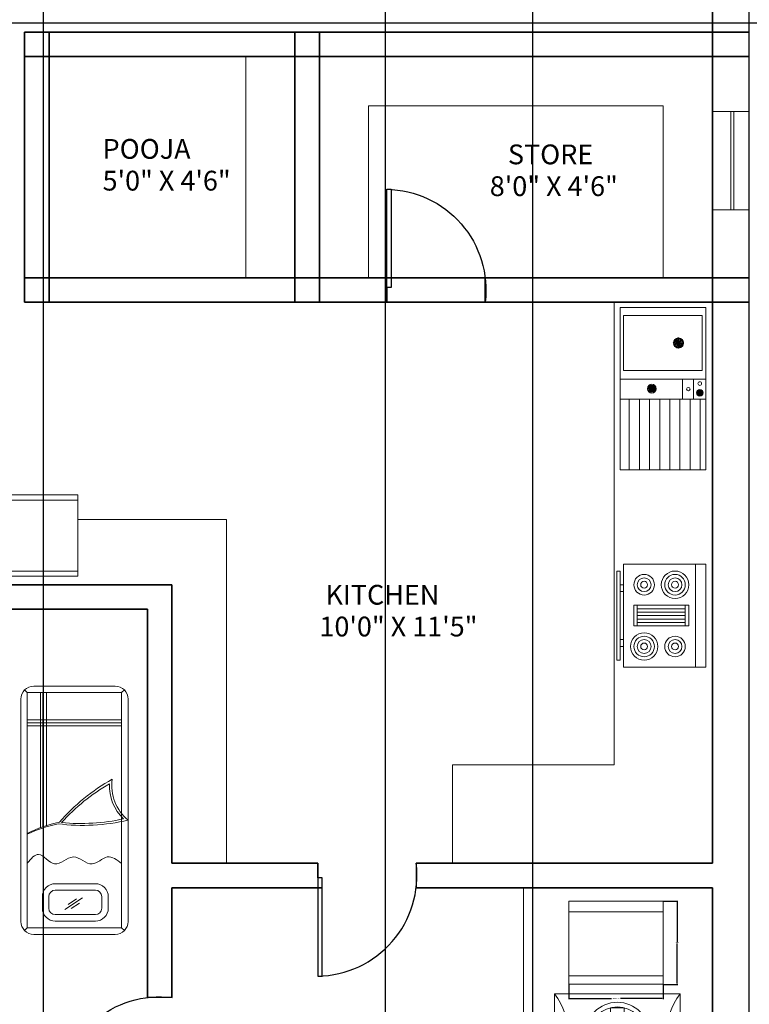
# Model space of a CAD drawing. Units: inches. Extents: x -61 to 1599, y -1316 to 257.
# Tile 94 of 204: x 367 to 545, y -407 to -166. Entities that reach past the tile are written whole.
import ezdxf

# ---------------------------------------------------------------- set-up
doc = ezdxf.new("R2010")
doc.units = ezdxf.units.IN
doc.header["$MEASUREMENT"] = 0
doc.linetypes.add('ACAD_ISO02W100', pattern=[15, 12, -3])
for name, color, linetype, lineweight in [('A-ANNO-DIMS', 2, 'Continuous', 18), ('A-AREA-IDEN', 1, 'Continuous', 18), ('A-EQPM', 9, 'Continuous', 18), ('A-FLOR-CASE', 8, 'Continuous', 18), ('A-FLOR-FIXT', 8, 'Continuous', 18), ('A-WALL-JAMB', 4, 'ACAD_ISO02W100', 25), ('DOORS', 2, 'Continuous', 25), ('FURNITURE', 83, 'Continuous', 18), ('WALLS', 4, 'Continuous', 35), ('WINDOWS', 220, 'Continuous', 18)]:
    doc.layers.add(name, color=color, linetype=linetype, lineweight=lineweight)
doc.layers.add('FUR', color=83, linetype='Continuous')
doc.styles.get("Standard").update_dxf_attribs({"font": 'arial.ttf'})
doc.dimstyles.get("Standard").update_dxf_attribs({"dimtxt": 0.18, "dimasz": 0.18, "dimexe": 0.18, "dimexo": 0.0625, "dimgap": 0.09, "dimtad": 0, "dimtih": 1, "dimtoh": 1, "dimdec": 0, "dimzin": 0, "dimdsep": 46, "dimlunit": 3, "dimtxsty": 'Standard', "dimcen": 0.09, "dimadec": 0, "dimazin": 0, "dimtfac": 1, "dimtdec": 0, "dimtofl": 0, "dimtmove": 0, "dimatfit": 3, "dimfxl": 1, "dimtolj": 1, "dimtzin": 0, "dimarcsym": 0})

# ---------------------------------------------------------------- blocks, each defined once
blk = doc.blocks.new('Range-Oven - 30 in top')
for p, q in [((0, -3), (30, -3)), ((12, -6), (18, -6)), ((13, -20), (13, -6)), ((14, -6), (14, -20)), ((15, -20), (15, -6)), ((16, -6), (16, -20)), ((17, -20), (17, -6)), ((18, -20), (12, -20)), ((6, -24), (6, -25)), ((8, -25), (8, -24)), ((22, -25), (22, -24)), ((24, -24), (24, -25))]:
    blk.add_line(p, q)
for points in [[(0, -24), (0, 0), (30, 0), (30, -24)], [(12, -21), (12, -5), (18, -5), (18, -21)], [(2, -26), (2, -25), (28, -25), (28, -26)]]:
    blk.add_lwpolyline(points, close=True)
for centre, radius in [((6, -9), 4), ((6, -9), 3), ((6, -9), 2), ((6, -9), 1), ((24, -9), 3), ((24, -9), 2), ((24, -9), 1), ((24, -18), 4), ((6, -18), 3), ((6, -18), 2), ((6, -18), 1), ((24, -18), 3), ((24, -18), 2), ((24, -18), 1)]:
    blk.add_circle(centre, radius)
blk = doc.blocks.new('DOOR-SWING-24')
blk.add_line((0, 0), (0, 3.6))
blk.add_lwpolyline([(0, 0), (0, -24), (1.05, -24), (1.05, 0)], close=True)
blk.add_arc((-0.44, 0.62), 24.62, 271.0259, 6.9559)
blk = doc.blocks.new('WIN-24IN')
for p, q in [((0, 4.5), (0, 9)), ((0, 9), (0, 0)), ((24, 9), (24, 0)), ((0, 5.19), (24, 5.19)), ((0, 4.5), (24, 4.5))]:
    blk.add_line(p, q)
blk = doc.blocks.new('*U268')
at = {"layer": 'FUR'}
blk.add_line((0.41, 1.36), (0.41, 0.68), dxfattribs=at)
blk.add_open_spline([(0.41, 1.36), (0.24, 1.25), (-0.09, 1.02), (0.41, 0.7), (0.83, 0.34), (0.55, 0.11), (0.41, 0)], degree=3, knots=[0, 0, 0, 0, 0.474547, 0.949094, 1.393355, 1.837616, 1.837616, 1.837616, 1.837616], dxfattribs=at)
blk = doc.blocks.new('*U269')
at = {"layer": 'FUR', "transparency": 16777216}
for p, rotation in [((531.82, -257.55), 308.5714285714286), ((532.89, -258.18), 51.42857142857144), ((532.03, -256.89), 257.1428571428571), ((533.36, -257.68), 102.8571428571428), ((532.68, -256.65), 205.7142857142857), ((533.27, -257), 154.2857142857143)]:
    blk.add_blockref('*U268', p, dxfattribs=dict(at, rotation=rotation))
blk.add_blockref('*U268', (532.2, -258.12), dxfattribs=at)
blk = doc.blocks.new('*U270')
at = {"layer": 'FUR'}
blk.add_line((0.74, 2.46), (0.74, 1.23), dxfattribs=at)
blk.add_open_spline([(0.74, 2.46), (0.44, 2.26), (-0.16, 1.84), (0.74, 1.26), (1.5, 0.61), (0.99, 0.2), (0.74, 0)], degree=3, knots=[0, 0, 0, 0, 0.85637, 1.712739, 2.514455, 3.316171, 3.316171, 3.316171, 3.316171], dxfattribs=at)
blk = doc.blocks.new('*U271')
at = {"layer": 'FUR', "transparency": 16777216}
for p, rotation in [((959.72, -464.77), 308.5714285714286), ((961.65, -465.92), 51.42857142857144), ((960.11, -463.59), 257.1428571428571), ((962.51, -465.02), 102.8571428571428), ((961.27, -463.15), 205.7142857142858), ((962.34, -463.79), 154.2857142857143)]:
    blk.add_blockref('*U270', p, dxfattribs=dict(at, rotation=rotation))
blk.add_blockref('*U270', (960.41, -465.81), dxfattribs=at)
blk = doc.blocks.new('*U266')
at = {"layer": 'FUR'}
blk.add_line((0.41, 1.36), (0.41, 0.68), dxfattribs=at)
blk.add_open_spline([(0.41, 1.36), (0.24, 1.25), (-0.09, 1.02), (0.41, 0.7), (0.83, 0.34), (0.55, 0.11), (0.41, 0)], degree=3, knots=[0, 0, 0, 0, 0.474547, 0.949094, 1.393355, 1.837616, 1.837616, 1.837616, 1.837616], dxfattribs=at)
blk = doc.blocks.new('*U267')
at = {"layer": 'FUR', "transparency": 16777216}
for p, rotation in [((531.82, -257.55), 308.5714285714286), ((532.89, -258.18), 51.42857142857144), ((532.03, -256.89), 257.1428571428571), ((533.36, -257.68), 102.8571428571428), ((532.68, -256.65), 205.7142857142857), ((533.27, -257), 154.2857142857143)]:
    blk.add_blockref('*U266', p, dxfattribs=dict(at, rotation=rotation))
blk.add_blockref('*U266', (532.2, -258.12), dxfattribs=at)
blk = doc.blocks.new('SINK-WITH-DRAINBOARD')
for p, q in [((14.29, 30.97), (14.29, 29.74)), ((0, 22.17), (20.98, 22.17)), ((15.24, 17.27), (15.24, 22.17)), ((17.97, 22.17), (17.97, 17.27)), ((7.79, 19.82), (7.79, 19.14)), ((0, 17.27), (20.98, 17.27)), ((2.27, 0), (2.27, 17.27)), ((4.74, 0), (4.74, 17.27)), ((7.21, 0), (7.21, 17.27)), ((9.69, 0), (9.69, 17.27)), ((12.16, 0), (12.16, 17.27)), ((14.63, 0), (14.63, 17.27)), ((17.1, 0), (17.1, 17.27)), ((19.48, 18.8), (19.48, 18.12)), ((19.58, 0), (19.58, 17.27))]:
    blk.add_line(p, q)
for points in [[(20.98, 0), (0, 0), (0, 39.63), (20.98, 39.63)], [(20.07, 24.22), (0.86, 24.22), (0.86, 37.7), (20.07, 37.7)]]:
    blk.add_lwpolyline(points, close=True)
for centre, radius in [((14.29, 30.97), 1.23), ((7.78, 19.81), 1.08), ((7.78, 19.81), 0.877), ((7.79, 19.82), 0.682), ((16.69, 19.72), 0.419), ((19.48, 18.8), 0.816), ((19.48, 18.8), 0.816), ((19.48, 18.8), 0.682), ((19.48, 21.05), 0.455)]:
    blk.add_circle(centre, radius)
for name, p in [('*U271', (-946.85, 495.54)), ('*U269', (-524.82, 277.26)), ('*U267', (-513.12, 276.24))]:
    blk.add_blockref(name, p)
blk = doc.blocks.new('WASHING-MACHINE')
for p, q in [((19.24, 4.47), (19.22, 15.41)), ((0.98, 10.64), (0.75, 10.64)), ((0.96, 11.16), (1.13, 11)), ((1.12, 10.28), (0.96, 10.12)), ((1.49, 11.38), (1.49, 11.15)), ((1.49, 10.12), (1.49, 9.89)), ((2.02, 11.15), (1.86, 10.99)), ((1.86, 10.28), (2.02, 10.12)), ((2.23, 10.64), (2, 10.64)), ((11, 9.47), (11, 11.68))]:
    blk.add_line(p, q)
for points in [[(30.68, 0), (0, 0), (0, 19.87), (30.68, 19.87)], [(16.98, 3.42), (13.7, 3.42), (13.7, 16.45), (16.98, 16.45)], [(20.43, 13.78), (18.01, 13.78), (18.01, 13.95), (20.43, 13.95)], [(18.09, 12.45), (20.41, 11.74), (20.35, 11.57), (18.04, 12.29)], [(18.21, 13.64), (20.52, 12.92), (20.47, 12.76), (18.16, 13.47)], [(18.22, 12.89), (20.53, 12.18), (20.48, 12.01), (18.17, 12.73)], [(20.44, 10.23), (18.02, 10.23), (18.02, 10.4), (20.44, 10.4)], [(18.1, 11.71), (20.41, 10.99), (20.36, 10.83), (18.05, 11.54)], [(18.22, 10.09), (20.53, 9.38), (20.48, 9.21), (18.17, 9.92)], [(18.1, 8.63), (20.42, 7.91), (20.37, 7.75), (18.05, 8.46)], [(18.11, 7.88), (20.42, 7.17), (20.37, 7), (18.06, 7.72)], [(18.23, 9.07), (20.54, 8.36), (20.49, 8.19), (18.18, 8.91)], [(20.45, 6.56), (18.03, 6.56), (18.03, 6.73), (20.45, 6.73)], [(18.23, 6.42), (20.54, 5.7), (20.49, 5.54), (18.18, 6.25)]]:
    blk.add_lwpolyline(points, close=True)
for centre, radius in [((15.34, 9.94), 7.85), ((15.34, 9.94), 7.85), ((15.34, 9.94), 6.71), ((1.28, 13.83), 0.526), ((10.77, 12.86), 0.381), ((10.77, 12.86), 0.289), ((1.49, 10.64), 0.742), ((1.49, 10.64), 0.513), ((1.49, 10.64), 0.178), ((1.49, 10.64), 0.07), ((1.28, 7.75), 0.526), ((10.77, 8.29), 0.381), ((10.77, 8.29), 0.289)]:
    blk.add_circle(centre, radius)
for centre, radius, start, end in [((-13.12, 9.94), 16.46, 322.8671, 37.1329), ((43.8, 9.94), 16.46, 142.8671, 217.1329), ((12.8, 10.57), 2.11, 148.4251, 211.5749), ((9.2, 10.57), 2.11, 328.4251, 31.5749)]:
    blk.add_arc(centre, radius, start, end)
blk = doc.blocks.new('UTILITY-CABINET')
for p, q in [((0, 17.69), (23.01, 17.69)), ((0, 2.1), (23.01, 2.1))]:
    blk.add_line(p, q)
blk.add_lwpolyline([(23.01, 0), (0, 0), (0, 20.31), (23.01, 20.31)], close=True)
blk = doc.blocks.new('KITCHEN-BASE-UNIT')
for p, q in [((25.07, 18.6), (0, 18.6)), ((25.07, 1.23), (0, 1.23))]:
    blk.add_line(p, q)
blk.add_lwpolyline([(25.07, 0), (0, 0), (0, 19.92), (25.07, 19.92)], close=True)
blk = doc.blocks.new('STORE-SHELVING')
for p, q in [((0, 42), (72, 42)), ((0, 12), (0, 42)), ((72, 42), (72, 12)), ((0, 0), (0, 12)), ((72, 0), (72, 12))]:
    blk.add_line(p, q)
blk = doc.blocks.new('*D658')
at = {"layer": 'A-ANNO-DIMS', "color": 0, "lineweight": -2, "transparency": 16777216}
for p, q in [((500.63, -401.98), (500.63, -405.55)), ((523.64, -401.98), (523.64, -405.55)), ((500.81, -405.37), (511.03, -405.37)), ((523.46, -405.37), (513.24, -405.37))]:
    blk.add_line(p, q, dxfattribs=at)
at = {"layer": 'A-ANNO-DIMS', "color": 0, "transparency": 16777216}
for points in [[(500.81, -405.34), (500.81, -405.4), (500.63, -405.37)], [(523.46, -405.34), (523.46, -405.4), (523.64, -405.37)]]:
    blk.add_solid(points, dxfattribs=at)
at = {"layer": 'DEFPOINTS', "color": 0, "transparency": 16777216}
for p in [(500.63, -401.92), (523.64, -401.92), (523.64, -405.37)]:
    blk.add_point(p, dxfattribs=at)
at = {"layer": 'A-ANNO-DIMS', "color": 0, "transparency": 16777216, "insert": (512.14, -405.37), "char_height": 0.18, "attachment_point": 5}
blk.add_mtext('\\A1;CABINET 23 TYP.', dxfattribs=at)
blk = doc.blocks.new('*D659')
at = {"layer": 'A-ANNO-DIMS', "color": 0, "lineweight": -2, "transparency": 16777216}
for p, q in [((523.7, -381.61), (527.27, -381.61)), ((527.09, -381.79), (527.09, -391.58)), ((527.09, -401.74), (527.09, -391.94)), ((523.7, -401.92), (527.27, -401.92))]:
    blk.add_line(p, q, dxfattribs=at)
at = {"layer": 'A-ANNO-DIMS', "color": 0, "transparency": 16777216}
for points in [[(527.06, -381.79), (527.12, -381.79), (527.09, -381.61)], [(527.06, -401.74), (527.12, -401.74), (527.09, -401.92)]]:
    blk.add_solid(points, dxfattribs=at)
at = {"layer": 'DEFPOINTS', "color": 0, "transparency": 16777216}
for p in [(523.64, -381.61), (527.09, -381.61), (523.64, -401.92)]:
    blk.add_point(p, dxfattribs=at)
at = {"layer": 'A-ANNO-DIMS', "color": 0, "transparency": 16777216, "insert": (527.09, -391.76), "char_height": 0.18, "attachment_point": 5}
blk.add_mtext('\\A1;20 TYP.', dxfattribs=at)
blk = doc.blocks.new('*D699')
at = {"layer": 'A-ANNO-DIMS', "color": 0, "lineweight": -2, "transparency": 16777216}
for p, q in [((835.64, -167.17), (-61.08, -167.17)), ((-60.9, -167.35), (-60.9, -306.73)), ((-60.9, -446.47), (-60.9, -307.09)), ((841.64, -446.65), (-61.08, -446.65))]:
    blk.add_line(p, q, dxfattribs=at)
at = {"layer": 'A-ANNO-DIMS', "color": 0, "transparency": 16777216}
for points in [[(-60.93, -167.35), (-60.87, -167.35), (-60.9, -167.17)], [(-60.93, -446.47), (-60.87, -446.47), (-60.9, -446.65)]]:
    blk.add_solid(points, dxfattribs=at)
at = {"layer": 'DEFPOINTS', "color": 0, "transparency": 16777216}
for p in [(835.7, -167.17), (-60.9, -446.65), (841.7, -446.65)]:
    blk.add_point(p, dxfattribs=at)
at = {"layer": 'A-ANNO-DIMS', "color": 0, "transparency": 16777216, "insert": (-60.9, -306.91), "char_height": 0.18, "attachment_point": 5}
blk.add_mtext('\\A1;279.5', dxfattribs=at)
blk = doc.blocks.new('*D703')
at = {"layer": 'A-ANNO-DIMS', "color": 0, "lineweight": -2, "transparency": 16777216}
for p, q in [((372.32, -616.88), (372.32, 257.46)), ((455.83, -616.88), (455.83, 257.46)), ((372.5, 257.28), (413.7, 257.28)), ((455.65, 257.28), (414.45, 257.28))]:
    blk.add_line(p, q, dxfattribs=at)
at = {"layer": 'A-ANNO-DIMS', "color": 0, "transparency": 16777216}
for points in [[(372.5, 257.31), (372.5, 257.25), (372.32, 257.28)], [(455.65, 257.31), (455.65, 257.25), (455.83, 257.28)]]:
    blk.add_solid(points, dxfattribs=at)
at = {"layer": 'DEFPOINTS', "color": 0, "transparency": 16777216}
for p in [(455.83, 257.28), (372.32, -616.94), (455.83, -616.94)]:
    blk.add_point(p, dxfattribs=at)
at = {"layer": 'A-ANNO-DIMS', "color": 0, "transparency": 16777216, "insert": (414.08, 257.28), "char_height": 0.18, "attachment_point": 5}
blk.add_mtext('\\A1;83.51', dxfattribs=at)
blk = doc.blocks.new('*D704')
at = {"layer": 'A-ANNO-DIMS', "color": 0, "lineweight": -2, "transparency": 16777216}
for p, q in [((491.83, -616.88), (491.83, 257.46)), ((544.7, -616.88), (544.7, 257.46)), ((492.01, 257.28), (517.87, 257.28)), ((544.52, 257.28), (518.66, 257.28))]:
    blk.add_line(p, q, dxfattribs=at)
at = {"layer": 'A-ANNO-DIMS', "color": 0, "transparency": 16777216}
for points in [[(492.01, 257.31), (492.01, 257.25), (491.83, 257.28)], [(544.52, 257.31), (544.52, 257.25), (544.7, 257.28)]]:
    blk.add_solid(points, dxfattribs=at)
at = {"layer": 'DEFPOINTS', "color": 0, "transparency": 16777216}
for p in [(544.7, 257.28), (491.83, -616.94), (544.7, -616.94)]:
    blk.add_point(p, dxfattribs=at)
at = {"layer": 'A-ANNO-DIMS', "color": 0, "transparency": 16777216, "insert": (518.27, 257.28), "char_height": 0.18, "attachment_point": 5}
blk.add_mtext('\\A1;52.87', dxfattribs=at)

msp = doc.modelspace()

# ---------------------------------------------------------------- linework, layer by layer
at = {"layer": 'A-FLOR-CASE'}
for p, q in [((535.7028, -222.7455), (535.7028, -222.7455)), ((511.7028, -235.3229), (511.7028, -259.3229)), ((511.7028, -348.3229), (511.7028, -259.3229)), ((380.7476, -288.4105), (417.0519, -288.4105)), ((417.0519, -288.4105), (417.0519, -372.3229)), ((511.7028, -348.3229), (472.2349, -348.3229)), ((472.2349, -348.3229), (472.2349, -372.3229)), ((489.5747, -432.3229), (489.5747, -378.3229))]:
    msp.add_line(p, q, dxfattribs=at)
msp.add_lwpolyline([(433.7028, -229.3229), (421.7505, -229.3229), (421.7505, -175.3229), (433.7028, -175.3229)], close=True, dxfattribs=at)
at = {"layer": 'A-WALL-JAMB'}
for p, q in [((456.2028, -235.3229), (456.2028, -229.3229)), ((480.2028, -235.3229), (480.1983, -229.3229)), ((439.3522, -372.3229), (439.3522, -378.3229)), ((463.3522, -372.3229), (463.3522, -378.3229)), ((403.7028, -405.1414), (397.7028, -405.1458))]:
    msp.add_line(p, q, dxfattribs=at)
at = {"layer": 'FURNITURE'}
for p, q in [((368.3698, -330.6674), (367.7148, -330.0124)), ((371.5985, -363.6544), (371.5985, -330.6674)), ((372.1865, -363.443), (372.1865, -330.6674)), ((373.0588, -363.1542), (373.0588, -330.6674)), ((391.4076, -330.6674), (392.0626, -330.0124)), ((391.4076, -337.3084), (368.3698, -337.3084)), ((391.4076, -338.0177), (368.3698, -338.0177)), ((391.4076, -338.7871), (368.3698, -338.7871)), ((381.8729, -380.7881), (377.5662, -383.6749)), ((378.3763, -382.3874), (380.413, -381.0304)), ((379.072, -383.4316), (381.1087, -382.0746)), ((368.3698, -388.1313), (367.7148, -388.7863)), ((392.0626, -388.7863), (391.4076, -388.1313))]:
    msp.add_line(p, q, dxfattribs=at)
for points in [[(369.9511, -329.0861), (389.8263, -329.0861, -0.41421356), (392.989, -332.2487), (392.989, -386.55, -0.41421356), (389.8263, -389.7126), (369.9511, -389.7126, -0.41421356), (366.7885, -386.55), (366.7885, -332.2487, -0.41421356)], [(375.197, -377.3355), (384.9839, -377.3355, -0.41421356), (388.1465, -380.4982), (388.1465, -383.3141, -0.41421356), (384.9839, -386.4767), (375.197, -386.4767, -0.41421356), (372.0344, -383.3141), (372.0344, -380.4982, -0.41421356)], [(375.197, -378.9168), (384.9839, -378.9168, -0.41421356), (386.5652, -380.4982), (386.5652, -383.3141, -0.41421356), (384.9839, -384.8954), (375.197, -384.8954, -0.41421356), (373.6157, -383.3141), (373.6157, -380.4982, -0.41421356)]]:
    msp.add_lwpolyline(points, format="xyb", close=True, dxfattribs=at)
msp.add_lwpolyline([(368.3698, -330.6674), (391.4076, -330.6674), (391.4076, -388.1313), (368.3698, -388.1313)], close=True, dxfattribs=at)
for centre, radius, start, end in [((412.8702, -394.1626), 48.5558, 119.302799, 139.065497), ((412.7906, -394.9259), 48.5558, 120.122754, 137.951503), ((399.4118, -353.4771), 11.0029, 177.136894, 226.788842), ((400.0028, -353.343), 11.0029, 172.042189, 230.397858), ((382.2263, -392.3018), 30.5553, 101.397161, 116.967867), ((381.9164, -392.6627), 30.5553, 101.397161, 116.317614), ((381.953, -314.5357), 48.5558, 262.813151, 283.137248), ((381.4332, -314.0773), 48.5558, 264.446321, 282.422187)]:
    msp.add_arc(centre, radius, start, end, dxfattribs=at)
msp.add_open_spline([(391.4076, -372.395), (390.2379, -371.5093), (387.818, -369.677), (383.9669, -374.1451), (379.6119, -368.943), (375.0321, -374.5225), (371.3585, -368.6867), (369.2784, -371.2237), (368.3698, -372.3318)], degree=3, knots=[0, 0, 0, 0, 3.84254534, 7.94890144, 12.81558195, 17.74158221, 22.25649, 25.75782552, 25.75782552, 25.75782552, 25.75782552], dxfattribs=at)
at = {"layer": 'WALLS'}
for p, q in [((535.7028, -13.3229), (535.7028, -175.3229)), ((367.7028, -169.3229), (403.7028, -169.3229)), ((367.7028, -235.3229), (367.7028, -169.3229)), ((373.7028, -235.3229), (373.7028, -169.3229)), ((397.7028, -169.3229), (544.7028, -169.3229)), ((433.7028, -235.3229), (433.7028, -169.3229)), ((439.7028, -235.3229), (439.7028, -169.3229)), ((367.7028, -175.3229), (373.7028, -175.3229)), ((373.7028, -175.3229), (433.7028, -175.3229)), ((433.7028, -175.3229), (439.7028, -175.3229)), ((439.7028, -175.3229), (535.7028, -175.3229)), ((535.7028, -282.3229), (535.7028, -175.3229)), ((535.7028, -175.3229), (544.7028, -175.3229)), ((367.7028, -229.3229), (544.7028, -229.3229)), ((433.7028, -229.3229), (544.7028, -229.3229)), ((367.7028, -235.3229), (544.7028, -235.3229)), ((433.7028, -235.3229), (544.7028, -235.3229)), ((535.7028, -282.3229), (535.7028, -372.3229)), ((325.7028, -304.3229), (403.7028, -304.3229)), ((403.7028, -304.3229), (403.7028, -372.3229)), ((325.7028, -310.3229), (397.7028, -310.3229)), ((397.7028, -310.3229), (397.7028, -405.1458)), ((403.7028, -372.3229), (439.3522, -372.3229)), ((463.3522, -372.3229), (535.7028, -372.3229)), ((403.7028, -378.3229), (440.4022, -378.3229)), ((403.7028, -378.3229), (403.7028, -405.1414)), ((463.3477, -378.3229), (535.7028, -378.3229)), ((535.7028, -378.3229), (535.7028, -432.3229))]:
    msp.add_line(p, q, dxfattribs=at)

# ---------------------------------------------------------------- block references
at = {"layer": 'A-EQPM', "xscale": 0.8378013827109642, "yscale": 0.8378013827109642, "zscale": 0.8378013827109642, "rotation": 270}
msp.add_blockref('Range-Oven - 30 in top', (534.1022, -299.295), dxfattribs=at)
at = {"layer": 'A-EQPM'}
msp.add_blockref('WASHING-MACHINE', (497.133, -424.099), dxfattribs=at)
at = {"layer": 'A-FLOR-CASE'}
for name, p in [('STORE-SHELVING', (451.703, -229.323)), ('KITCHEN-BASE-UNIT', (355.674, -302.245)), ('UTILITY-CABINET', (500.634, -401.916))]:
    msp.add_blockref(name, p, dxfattribs=at)
at = {"layer": 'A-FLOR-FIXT'}
msp.add_blockref('SINK-WITH-DRAINBOARD', (513.125, -276.244), dxfattribs=at)
at = {"layer": 'DOORS', "extrusion": (0, 0, -1), "zscale": -1}
for p, rotation in [((-456.2028, -231.7229), 180), ((-400.1028, -429.1414), 89.99999999999973)]:
    msp.add_blockref('DOOR-SWING-24', p, dxfattribs=dict(at, rotation=rotation))
at = {"layer": 'DOORS'}
msp.add_blockref('DOOR-SWING-24', (439.3522, -375.9229), dxfattribs=at)
at = {"layer": 'WINDOWS', "rotation": 269.9999999999998}
msp.add_blockref('WIN-24IN', (535.7027, -188.7656), dxfattribs=at)

# ---------------------------------------------------------------- texts
at = {"layer": 'A-AREA-IDEN'}
for s, height, p in [('POOJA', 4.8321, (386.7531, -200.2805)), ('   STORE', 4.8321, (481.3179, -201.6263)), ('5\'0" X 4\'6"', 4.832098, (386.7531, -208.0429)), ('8\'0" X 4\'6"', 4.832098, (481.3179, -209.3886)), (' KITCHEN', 4.8321, (439.7144, -309.1831)), ('10\'0" X 11\'5"', 4.832098, (439.7144, -316.9454))]:
    msp.add_text(s, height=height, dxfattribs=at).set_placement(p)

# ---------------------------------------------------------------- dimensions: what is measured, and where the dimension line sits
at = {"layer": 'A-ANNO-DIMS'}
for base, p1, p2, picture, middle in [((455.8327, 257.2771), (372.3201, -616.9446), (455.8327, -616.9446), '*D703', (414.0764, 257.2771)), ((544.7028, 257.2771), (491.8327, -616.9446), (544.7028, -616.9446), '*D704', (518.2677, 257.2771))]:
    dim = msp.add_linear_dim(base=base, p1=p1, p2=p2, dimstyle='Standard', override={"dimdec": 2, "dimlfac": 1, "dimrnd": 0, "dimzin": 0, "dimdsep": 46, "dimlunit": 2}, dxfattribs=at)
    dim.commit()
    dim.dimension.update_dxf_attribs({"geometry": picture, "text_midpoint": middle})
dim = msp.add_linear_dim(base=(-60.8972, -446.6462), p1=(835.7028, -167.169), p2=(841.7028, -446.6462), angle=90, dimstyle='Standard', override={"dimdec": 1, "dimlfac": 1, "dimrnd": 0, "dimzin": 0, "dimdsep": 46, "dimlunit": 2}, dxfattribs=at)
dim.commit()
dim.dimension.update_dxf_attribs({"geometry": '*D699', "text_midpoint": (-60.8972, -306.9076)})
dim = msp.add_linear_dim(base=(527.0928, -381.606), p1=(523.6417, -401.9162), p2=(523.6417, -381.606), angle=90, text='<> TYP.', dimstyle='Standard', override={"dimdec": 0, "dimlfac": 1, "dimrnd": 0, "dimzin": 0, "dimdsep": 46, "dimlunit": 2}, dxfattribs=at)
dim.commit()
dim.dimension.update_dxf_attribs({"geometry": '*D659', "text_midpoint": (527.0928, -391.7611)})
dim = msp.add_linear_dim(base=(523.6417, -405.3673), p1=(500.6345, -401.9162), p2=(523.6417, -401.9162), text='CABINET <> TYP.', dimstyle='Standard', override={"dimdec": 0, "dimlfac": 1, "dimrnd": 0, "dimzin": 0, "dimdsep": 46, "dimlunit": 2}, dxfattribs=at)
dim.commit()
dim.dimension.update_dxf_attribs({"geometry": '*D658', "text_midpoint": (512.1381, -405.3673)})

doc.saveas('drawing.dxf')
